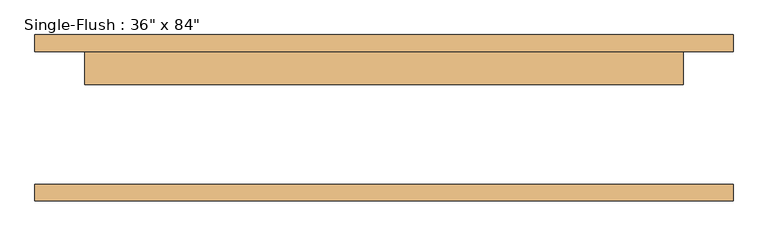
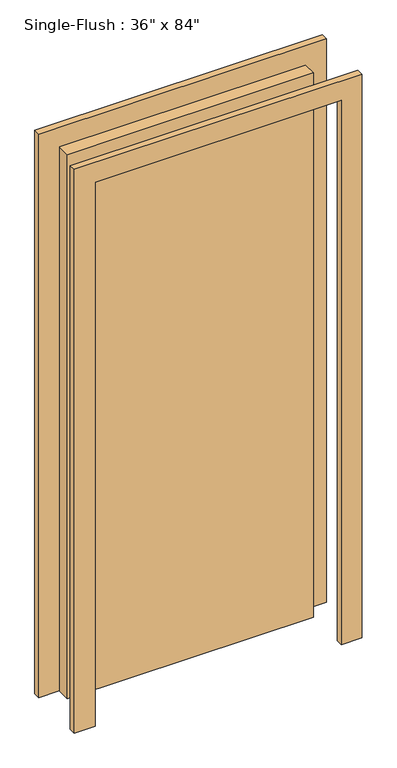
"""IFC4 building model written with IfcOpenShell, lengths in millimetres: door geometry."""

from ifc_helpers import new_model, si_unit, frame, origin, origin_with_axes, place, context, project, spatial, polyline, outline, extrude, source, transform, mapped, element, save


def door_54dd4da4(model_context):
    return source(origin(), model_context, "Body", "SweptSolid", [
        extrude(outline(polyline([(2209.8, -533.4), (0.0, -533.4), (0.0, -457.2), (2133.6, -457.2), (2133.6, 457.2), (0.0, 457.2), (0.0, 533.4), (2209.8, 533.4), (2209.8, -533.4)])), frame((0.0, 101.6, 0.0), z_axis=(0.0, 1.0, 0.0), x_axis=(0.0, 0.0, 1.0)), (0.0, 0.0, 1.0), 25.4),
        extrude(outline(polyline([(2209.8, 533.4), (2209.8, -533.4), (0.0, -533.4), (0.0, -457.2), (2133.6, -457.2), (2133.6, 457.2), (0.0, 457.2), (0.0, 533.4), (2209.8, 533.4)])), frame((0.0, -127.0, 0.0), z_axis=(0.0, 1.0, 0.0), x_axis=(0.0, 0.0, 1.0)), (0.0, 0.0, 1.0), 25.4),
        extrude(outline(polyline([(457.2, 50.8), (-457.2, 50.8), (-457.2, 101.6), (457.2, 101.6), (457.2, 50.8)])), origin_with_axes(), (0.0, 0.0, 1.0), 2133.6),
    ])


if __name__ == "__main__":
    model = new_model("IFC4")
    model_context = context("Model", 3, world=origin())
    ifc_project = project(units=[si_unit("LENGTHUNIT", "METRE", prefix="MILLI")], contexts=[model_context])
    site = spatial("IfcSite", under=ifc_project)
    building = spatial("IfcBuilding", under=site)
    placement = place(None, origin())
    door_shape = door_54dd4da4(model_context)
    element("IfcDoor", 1, ObjectType="Single-Flush : 36\" x 84\"", at=placement, inside=building, context=model_context, shape_type="MappedRepresentation", body=[
        mapped(door_shape, transform((0.0, 0.0, 0.0), x_axis=(1.0, 0.0, 0.0), y_axis=(0.0, 1.0, 0.0), z_axis=(0.0, 0.0, 1.0))),
    ])
    save(model, "model.ifc")

# Revit data of these elements
# Type "Single-Flush : 36\" x 84\""
#   Type Mark = "1"
#   Construction Type Id = "MDOOR"
#   Assembly Code = "C1020"
#   Analytic Construction = "Metal"
#   Thickness = 0' - 2"
#   Heat Transfer Coefficient (U) = 0.651978 BTU/(h·ft²·°F)
#   Height = 7' - 0"
#   Trim Projection Ext = 0' - 1"
#   Trim Projection Int = 0' - 1"
#   Trim Width = 0' - 3"
#   Width = 3' - 0"
#   Define Thermal Properties by = 1
#   Define Thermal Properties by = 1
#   Door Material = Door - Panel
#   Frame Material = Door - Frame
#   Visual Light Transmittance = 0
#   Solar Heat Gain Coefficient = 0
#   Function = (empty or 0)
#   Wall Closure = (empty or 0)
# Element 1 (IfcDoor, "Single-Flush : 36\" x 84\"")
#   Materials on its faces: "Door - Frame", "Door - Panel"
# Materials
#   "Door - Panel": class "Wood", colour RGB 210 159 95, transparency 0, Cost = 0
#   "Door - Frame": colour RGB 118 70 51, transparency 0, Cost = 0
